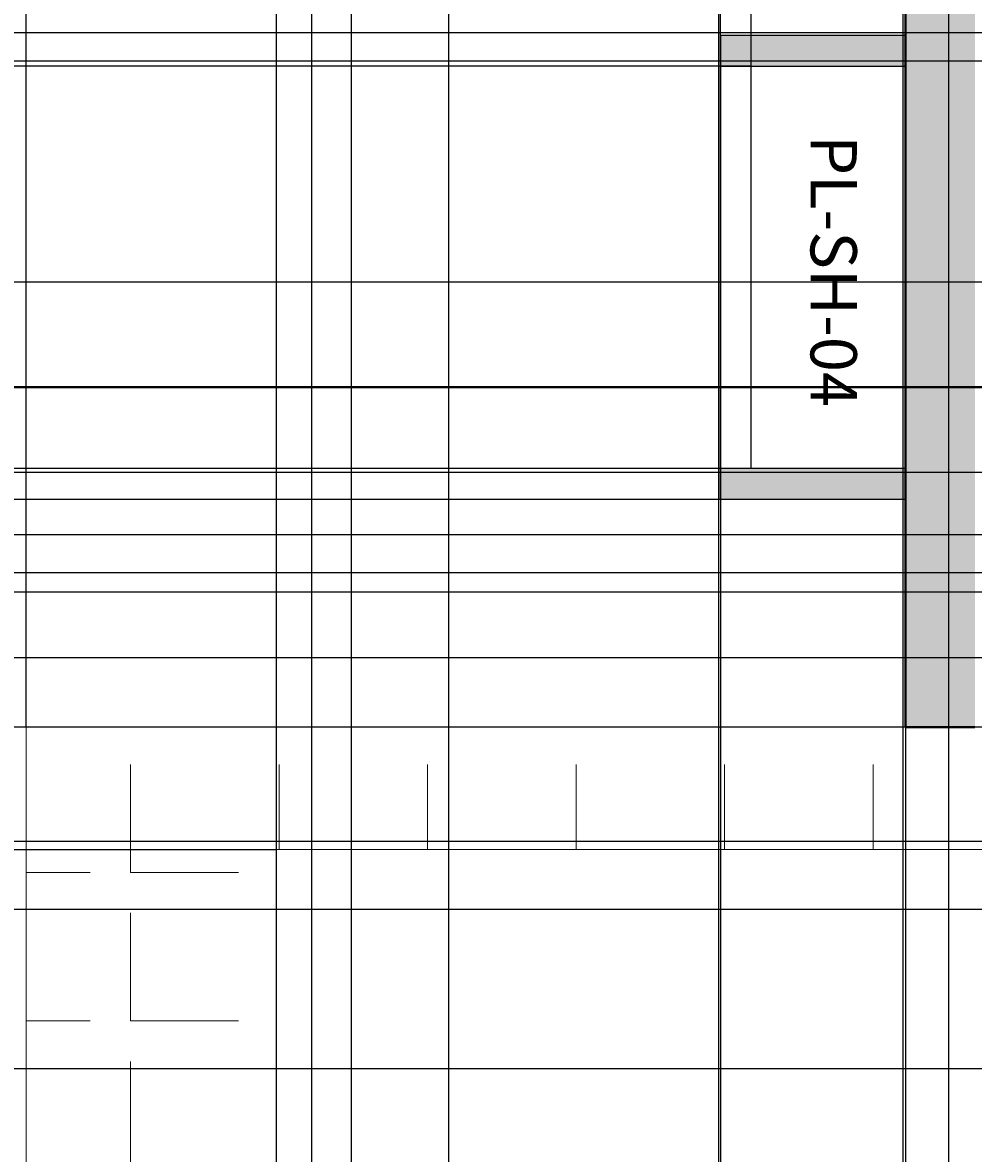
# Model space of a CAD drawing. Units: inches. Extents: x 818 to 1898, y 976 to 2364.
# Tile 7 of 96: x 1083 to 1207, y 1446 to 1592. Entities that reach past the tile are written whole.
import ezdxf

# ---------------------------------------------------------------- set-up
doc = ezdxf.new("R2010")
doc.units = ezdxf.units.IN
doc.header["$LTSCALE"] = 5
doc.header["$MEASUREMENT"] = 0
for name, color, linetype, lineweight in [('A-ANNO-DIMS', 2, 'Continuous', 18), ('A-ANNO-TEXT', 7, 'Continuous', 18), ('A-FLOR-SHFT', 7, 'Continuous', 25), ('A-WALL', 7, 'Continuous', 40), ('C-PKNG', 8, 'Continuous', 18), ('C-PKNG-PATT', 9, 'Continuous', 9), ('L-PLNT-BEDS', 94, 'Continuous', 18)]:
    doc.layers.add(name, color=color, linetype=linetype, lineweight=lineweight)
doc.layers.add('A-WALL-PATT', color=251, linetype='Continuous', lineweight=13, true_color=0x636466)
doc.styles.get("Standard").update_dxf_attribs({"font": 'arial.ttf'})
doc.dimstyles.get("Standard").update_dxf_attribs({"dimtxt": 0.18, "dimasz": 0.18, "dimexe": 0.18, "dimexo": 0.0625, "dimgap": 0.09, "dimtad": 0, "dimtih": 1, "dimtoh": 1, "dimdec": 4, "dimzin": 0, "dimdsep": 46, "dimtxsty": 'Standard', "dimcen": 0.09, "dimadec": 0, "dimazin": 0, "dimtfac": 1, "dimtdec": 4, "dimtofl": 0, "dimtmove": 0, "dimatfit": 3, "dimfxl": 1, "dimtolj": 1, "dimtzin": 0, "dimarcsym": 0})
pattern_1 = [(0, (0, 0), (0, 19.25), [14, -5.25]), (90, (0, 0), (-19.25, 1e-15), [14, -5.25])]

# ---------------------------------------------------------------- blocks, each defined once
blk = doc.blocks.new('*D59')
at = {"layer": 'A-ANNO-DIMS', "color": 0, "lineweight": -2, "ltscale": 5, "transparency": 16777216}
for p, q in [((1251.64, 2300.39), (818.03, 2300.39)), ((818.21, 2300.21), (818.21, 1669.95)), ((818.21, 1039.32), (818.21, 1669.59)), ((896.05, 1039.14), (818.03, 1039.14))]:
    blk.add_line(p, q, dxfattribs=at)
at = {"layer": 'A-ANNO-DIMS', "color": 0, "ltscale": 5, "transparency": 16777216}
for points in [[(818.18, 2300.21), (818.24, 2300.21), (818.21, 2300.39)], [(818.18, 1039.32), (818.24, 1039.32), (818.21, 1039.14)]]:
    blk.add_solid(points, dxfattribs=at)
at = {"layer": 'Defpoints', "color": 0, "ltscale": 5, "transparency": 16777216}
for p in [(818.21, 2300.39), (1251.71, 2300.39), (896.11, 1039.14)]:
    blk.add_point(p, dxfattribs=at)
at = {"layer": 'A-ANNO-DIMS', "color": 0, "ltscale": 5, "transparency": 16777216, "insert": (818.21, 1669.77), "char_height": 0.18, "attachment_point": 5}
blk.add_mtext('\\A1;1261.2', dxfattribs=at)
blk = doc.blocks.new('*D61')
at = {"layer": 'A-ANNO-DIMS', "color": 0, "lineweight": -2, "ltscale": 5, "transparency": 16777216}
for p, q in [((1071.73, 1203.03), (1071.73, 2363.87)), ((1071.91, 2363.69), (1250.94, 2363.69)), ((1430.55, 2363.69), (1251.51, 2363.69)), ((1430.73, 1203.03), (1430.73, 2363.87))]:
    blk.add_line(p, q, dxfattribs=at)
at = {"layer": 'A-ANNO-DIMS', "color": 0, "ltscale": 5, "transparency": 16777216}
for points in [[(1071.91, 2363.72), (1071.91, 2363.66), (1071.73, 2363.69)], [(1430.55, 2363.72), (1430.55, 2363.66), (1430.73, 2363.69)]]:
    blk.add_solid(points, dxfattribs=at)
at = {"layer": 'Defpoints', "color": 0, "ltscale": 5, "transparency": 16777216}
for p in [(1430.73, 2363.69), (1071.73, 1202.96), (1430.73, 1202.96)]:
    blk.add_point(p, dxfattribs=at)
at = {"layer": 'A-ANNO-DIMS', "color": 0, "ltscale": 5, "transparency": 16777216, "insert": (1251.23, 2363.69), "char_height": 0.18, "attachment_point": 5}
blk.add_mtext('\\A1;359', dxfattribs=at)
blk = doc.blocks.new('*D63')
at = {"layer": 'A-ANNO-DIMS', "color": 0, "lineweight": -2, "ltscale": 5, "transparency": 16777216}
for p, q in [((1116.13, 1485.2), (818.03, 1485.2)), ((818.21, 1485.02), (818.21, 1360.77)), ((818.21, 1236.14), (818.21, 1360.4)), ((1116.13, 1235.96), (818.03, 1235.96))]:
    blk.add_line(p, q, dxfattribs=at)
at = {"layer": 'A-ANNO-DIMS', "color": 0, "ltscale": 5, "transparency": 16777216}
for points in [[(818.18, 1485.02), (818.24, 1485.02), (818.21, 1485.2)], [(818.18, 1236.14), (818.24, 1236.14), (818.21, 1235.96)]]:
    blk.add_solid(points, dxfattribs=at)
at = {"layer": 'Defpoints', "color": 0, "ltscale": 5, "transparency": 16777216}
for p in [(818.21, 1485.2), (1116.19, 1485.2), (1116.19, 1235.96)]:
    blk.add_point(p, dxfattribs=at)
at = {"layer": 'A-ANNO-DIMS', "color": 0, "ltscale": 5, "transparency": 16777216, "insert": (818.21, 1360.58), "char_height": 0.18, "attachment_point": 5}
blk.add_mtext('\\A1;249.24', dxfattribs=at)
blk = doc.blocks.new('*D64')
at = {"layer": 'A-ANNO-DIMS', "color": 0, "lineweight": -2, "ltscale": 5, "transparency": 16777216}
for p, q in [((1197.73, 1501.14), (1197.73, 2363.87)), ((1197.91, 2363.69), (1313.93, 2363.69)), ((1430.55, 2363.69), (1314.52, 2363.69)), ((1430.73, 1501.14), (1430.73, 2363.87))]:
    blk.add_line(p, q, dxfattribs=at)
at = {"layer": 'A-ANNO-DIMS', "color": 0, "ltscale": 5, "transparency": 16777216}
for points in [[(1197.91, 2363.72), (1197.91, 2363.66), (1197.73, 2363.69)], [(1430.55, 2363.72), (1430.55, 2363.66), (1430.73, 2363.69)]]:
    blk.add_solid(points, dxfattribs=at)
at = {"layer": 'Defpoints', "color": 0, "ltscale": 5, "transparency": 16777216}
for p in [(1430.73, 2363.69), (1197.73, 1501.08), (1430.73, 1501.08)]:
    blk.add_point(p, dxfattribs=at)
at = {"layer": 'A-ANNO-DIMS', "color": 0, "ltscale": 5, "transparency": 16777216, "insert": (1314.23, 2363.69), "char_height": 0.18, "attachment_point": 5}
blk.add_mtext('\\A1;233', dxfattribs=at)
blk = doc.blocks.new('*D82')
at = {"layer": 'A-ANNO-DIMS', "color": 0, "lineweight": -2, "ltscale": 5, "transparency": 16777216}
for p, q in [((1083.73, 1501.14), (1083.73, 2363.87)), ((1083.91, 2363.69), (1140.45, 2363.69)), ((1197.55, 2363.69), (1141.01, 2363.69)), ((1197.73, 1501.14), (1197.73, 2363.87))]:
    blk.add_line(p, q, dxfattribs=at)
at = {"layer": 'A-ANNO-DIMS', "color": 0, "ltscale": 5, "transparency": 16777216}
for points in [[(1083.91, 2363.72), (1083.91, 2363.66), (1083.73, 2363.69)], [(1197.55, 2363.72), (1197.55, 2363.66), (1197.73, 2363.69)]]:
    blk.add_solid(points, dxfattribs=at)
at = {"layer": 'Defpoints', "color": 0, "ltscale": 5, "transparency": 16777216}
for p in [(1197.73, 2363.69), (1083.73, 1501.08), (1197.73, 1501.08)]:
    blk.add_point(p, dxfattribs=at)
at = {"layer": 'A-ANNO-DIMS', "color": 0, "ltscale": 5, "transparency": 16777216, "insert": (1140.73, 2363.69), "char_height": 0.18, "attachment_point": 5}
blk.add_mtext('\\A1;114', dxfattribs=at)
blk = doc.blocks.new('*D84')
at = {"layer": 'A-ANNO-DIMS', "color": 0, "lineweight": -2, "ltscale": 5, "transparency": 16777216}
for p, q in [((1197.66, 1700.08), (818.03, 1700.08)), ((818.21, 1699.9), (818.21, 1600.76)), ((818.21, 1501.26), (818.21, 1600.4)), ((1197.66, 1501.08), (818.03, 1501.08))]:
    blk.add_line(p, q, dxfattribs=at)
at = {"layer": 'A-ANNO-DIMS', "color": 0, "ltscale": 5, "transparency": 16777216}
for points in [[(818.18, 1699.9), (818.24, 1699.9), (818.21, 1700.08)], [(818.18, 1501.26), (818.24, 1501.26), (818.21, 1501.08)]]:
    blk.add_solid(points, dxfattribs=at)
at = {"layer": 'Defpoints', "color": 0, "ltscale": 5, "transparency": 16777216}
for p in [(818.21, 1700.08), (1197.73, 1700.08), (1197.73, 1501.08)]:
    blk.add_point(p, dxfattribs=at)
at = {"layer": 'A-ANNO-DIMS', "color": 0, "ltscale": 5, "transparency": 16777216, "insert": (818.21, 1600.58), "char_height": 0.18, "attachment_point": 5}
blk.add_mtext('\\A1;199', dxfattribs=at)
blk = doc.blocks.new('*D93')
at = {"layer": 'A-ANNO-DIMS', "color": 0, "lineweight": -2, "ltscale": 5, "transparency": 16777216}
for p, q in [((1068.34, 1071.12), (1068.34, 2363.87)), ((1068.52, 2363.69), (1094.16, 2363.69)), ((1120.58, 2363.69), (1094.94, 2363.69)), ((1120.76, 1071.12), (1120.76, 2363.87))]:
    blk.add_line(p, q, dxfattribs=at)
at = {"layer": 'A-ANNO-DIMS', "color": 0, "ltscale": 5, "transparency": 16777216}
for points in [[(1068.52, 2363.72), (1068.52, 2363.66), (1068.34, 2363.69)], [(1120.58, 2363.72), (1120.58, 2363.66), (1120.76, 2363.69)]]:
    blk.add_solid(points, dxfattribs=at)
at = {"layer": 'Defpoints', "color": 0, "ltscale": 5, "transparency": 16777216}
for p in [(1120.76, 2363.69), (1068.34, 1071.06), (1120.76, 1071.06)]:
    blk.add_point(p, dxfattribs=at)
at = {"layer": 'A-ANNO-DIMS', "color": 0, "ltscale": 5, "transparency": 16777216, "insert": (1094.55, 2363.69), "char_height": 0.18, "attachment_point": 5}
blk.add_mtext('\\A1;52.42', dxfattribs=at)
blk = doc.blocks.new('*D94')
at = {"layer": 'A-ANNO-DIMS', "color": 0, "lineweight": -2, "ltscale": 5, "transparency": 16777216}
for p, q in [((1120.76, 1071.12), (1120.76, 2363.87)), ((1120.94, 2363.69), (1146.76, 2363.69)), ((1173.36, 2363.69), (1147.55, 2363.69)), ((1173.54, 1071.12), (1173.54, 2363.87))]:
    blk.add_line(p, q, dxfattribs=at)
at = {"layer": 'A-ANNO-DIMS', "color": 0, "ltscale": 5, "transparency": 16777216}
for points in [[(1120.94, 2363.72), (1120.94, 2363.66), (1120.76, 2363.69)], [(1173.36, 2363.72), (1173.36, 2363.66), (1173.54, 2363.69)]]:
    blk.add_solid(points, dxfattribs=at)
at = {"layer": 'Defpoints', "color": 0, "ltscale": 5, "transparency": 16777216}
for p in [(1173.54, 2363.69), (1120.76, 1071.06), (1173.54, 1071.06)]:
    blk.add_point(p, dxfattribs=at)
at = {"layer": 'A-ANNO-DIMS', "color": 0, "ltscale": 5, "transparency": 16777216, "insert": (1147.15, 2363.69), "char_height": 0.18, "attachment_point": 5}
blk.add_mtext('\\A1;52.78', dxfattribs=at)
blk = doc.blocks.new('*D95')
at = {"layer": 'A-ANNO-DIMS', "color": 0, "lineweight": -2, "ltscale": 5, "transparency": 16777216}
for p, q in [((1173.54, 1071.12), (1173.54, 2363.87)), ((1173.72, 2363.69), (1201.29, 2363.69)), ((1229.47, 2363.69), (1201.9, 2363.69)), ((1229.65, 1071.12), (1229.65, 2363.87))]:
    blk.add_line(p, q, dxfattribs=at)
at = {"layer": 'A-ANNO-DIMS', "color": 0, "ltscale": 5, "transparency": 16777216}
for points in [[(1173.72, 2363.72), (1173.72, 2363.66), (1173.54, 2363.69)], [(1229.47, 2363.72), (1229.47, 2363.66), (1229.65, 2363.69)]]:
    blk.add_solid(points, dxfattribs=at)
at = {"layer": 'Defpoints', "color": 0, "ltscale": 5, "transparency": 16777216}
for p in [(1229.65, 2363.69), (1173.54, 1071.06), (1229.65, 1071.06)]:
    blk.add_point(p, dxfattribs=at)
at = {"layer": 'A-ANNO-DIMS', "color": 0, "ltscale": 5, "transparency": 16777216, "insert": (1201.59, 2363.69), "char_height": 0.18, "attachment_point": 5}
blk.add_mtext('\\A1;56.1', dxfattribs=at)
blk = doc.blocks.new('*D109')
at = {"layer": 'A-ANNO-DIMS', "color": 0, "lineweight": -2, "ltscale": 5, "transparency": 16777216}
for p, q in [((1125.92, 1410.12), (1125.92, 2363.87)), ((1126.1, 2363.69), (1164.25, 2363.69)), ((1203.15, 2363.69), (1165, 2363.69)), ((1203.33, 1409.91), (1203.33, 2363.87))]:
    blk.add_line(p, q, dxfattribs=at)
at = {"layer": 'A-ANNO-DIMS', "color": 0, "ltscale": 5, "transparency": 16777216}
for points in [[(1126.1, 2363.72), (1126.1, 2363.66), (1125.92, 2363.69)], [(1203.15, 2363.72), (1203.15, 2363.66), (1203.33, 2363.69)]]:
    blk.add_solid(points, dxfattribs=at)
at = {"layer": 'Defpoints', "color": 0, "ltscale": 5, "transparency": 16777216}
for p in [(1203.33, 2363.69), (1125.92, 1410.05), (1203.33, 1409.85)]:
    blk.add_point(p, dxfattribs=at)
at = {"layer": 'A-ANNO-DIMS', "color": 0, "ltscale": 5, "transparency": 16777216, "insert": (1164.62, 2363.69), "char_height": 0.18, "attachment_point": 5}
blk.add_mtext('\\A1;77.41', dxfattribs=at)
blk = doc.blocks.new('*D116')
at = {"layer": 'A-ANNO-DIMS', "color": 0, "lineweight": -2, "ltscale": 5, "transparency": 16777216}
for p, q in [((1766.29, 1456.81), (818.03, 1456.81)), ((818.21, 1456.63), (818.21, 1417.41)), ((818.21, 1377.84), (818.21, 1417.05)), ((1766.29, 1377.66), (818.03, 1377.66))]:
    blk.add_line(p, q, dxfattribs=at)
at = {"layer": 'A-ANNO-DIMS', "color": 0, "ltscale": 5, "transparency": 16777216}
for points in [[(818.18, 1456.63), (818.24, 1456.63), (818.21, 1456.81)], [(818.18, 1377.84), (818.24, 1377.84), (818.21, 1377.66)]]:
    blk.add_solid(points, dxfattribs=at)
at = {"layer": 'Defpoints', "color": 0, "ltscale": 5, "transparency": 16777216}
for p in [(818.21, 1456.81), (1766.35, 1456.81), (1766.35, 1377.66)]:
    blk.add_point(p, dxfattribs=at)
at = {"layer": 'A-ANNO-DIMS', "color": 0, "ltscale": 5, "transparency": 16777216, "insert": (818.21, 1417.23), "char_height": 0.18, "attachment_point": 5}
blk.add_mtext('\\A1;79.15', dxfattribs=at)
blk = doc.blocks.new('*D117')
at = {"layer": 'A-ANNO-DIMS', "color": 0, "lineweight": -2, "ltscale": 5, "transparency": 16777216}
for p, q in [((1766.29, 1545.18), (818.03, 1545.18)), ((818.21, 1545), (818.21, 1501.18)), ((818.21, 1456.99), (818.21, 1500.81)), ((1766.29, 1456.81), (818.03, 1456.81))]:
    blk.add_line(p, q, dxfattribs=at)
at = {"layer": 'A-ANNO-DIMS', "color": 0, "ltscale": 5, "transparency": 16777216}
for points in [[(818.18, 1545), (818.24, 1545), (818.21, 1545.18)], [(818.18, 1456.99), (818.24, 1456.99), (818.21, 1456.81)]]:
    blk.add_solid(points, dxfattribs=at)
at = {"layer": 'Defpoints', "color": 0, "ltscale": 5, "transparency": 16777216}
for p in [(818.21, 1545.18), (1766.35, 1545.18), (1766.35, 1456.81)]:
    blk.add_point(p, dxfattribs=at)
at = {"layer": 'A-ANNO-DIMS', "color": 0, "ltscale": 5, "transparency": 16777216, "insert": (818.21, 1501), "char_height": 0.18, "attachment_point": 5}
blk.add_mtext('\\A1;88.37', dxfattribs=at)
blk = doc.blocks.new('*D118')
at = {"layer": 'A-ANNO-DIMS', "color": 0, "lineweight": -2, "ltscale": 5, "transparency": 16777216}
for p, q in [((1766.29, 1627.51), (818.03, 1627.51)), ((818.21, 1627.33), (818.21, 1586.53)), ((818.21, 1545.36), (818.21, 1586.16)), ((1766.29, 1545.18), (818.03, 1545.18))]:
    blk.add_line(p, q, dxfattribs=at)
at = {"layer": 'A-ANNO-DIMS', "color": 0, "ltscale": 5, "transparency": 16777216}
for points in [[(818.18, 1627.33), (818.24, 1627.33), (818.21, 1627.51)], [(818.18, 1545.36), (818.24, 1545.36), (818.21, 1545.18)]]:
    blk.add_solid(points, dxfattribs=at)
at = {"layer": 'Defpoints', "color": 0, "ltscale": 5, "transparency": 16777216}
for p in [(818.21, 1627.51), (1766.35, 1627.51), (1766.35, 1545.18)]:
    blk.add_point(p, dxfattribs=at)
at = {"layer": 'A-ANNO-DIMS', "color": 0, "ltscale": 5, "transparency": 16777216, "insert": (818.21, 1586.34), "char_height": 0.18, "attachment_point": 5}
blk.add_mtext('\\A1;82.32', dxfattribs=at)
blk = doc.blocks.new('*D122')
at = {"layer": 'A-ANNO-DIMS', "color": 0, "lineweight": -2, "ltscale": 5, "transparency": 16777216}
for p, q in [((1138.5, 1794.37), (1138.5, 975.66)), ((1071.73, 1688.02), (1071.73, 975.66)), ((1071.91, 975.84), (1104.72, 975.84)), ((1138.32, 975.84), (1105.51, 975.84))]:
    blk.add_line(p, q, dxfattribs=at)
at = {"layer": 'A-ANNO-DIMS', "color": 0, "ltscale": 5, "transparency": 16777216}
for points in [[(1071.91, 975.87), (1071.91, 975.81), (1071.73, 975.84)], [(1138.32, 975.87), (1138.32, 975.81), (1138.5, 975.84)]]:
    blk.add_solid(points, dxfattribs=at)
at = {"layer": 'Defpoints', "color": 0, "ltscale": 5, "transparency": 16777216}
for p in [(1138.5, 1794.43), (1071.73, 1688.08), (1138.5, 975.84)]:
    blk.add_point(p, dxfattribs=at)
at = {"layer": 'A-ANNO-DIMS', "color": 0, "ltscale": 5, "transparency": 16777216, "insert": (1105.11, 975.84), "char_height": 0.18, "attachment_point": 5}
blk.add_mtext('\\A1;66.78', dxfattribs=at)
blk = doc.blocks.new('*D126')
at = {"layer": 'A-ANNO-DIMS', "color": 0, "lineweight": -2, "ltscale": 5, "transparency": 16777216}
for p, q in [((1035.38, 1252.09), (1035.38, 2363.87)), ((1035.56, 2363.69), (1075.41, 2363.69)), ((1116.01, 2363.69), (1076.16, 2363.69)), ((1116.19, 1236.03), (1116.19, 2363.87))]:
    blk.add_line(p, q, dxfattribs=at)
at = {"layer": 'A-ANNO-DIMS', "color": 0, "ltscale": 5, "transparency": 16777216}
for points in [[(1035.56, 2363.72), (1035.56, 2363.66), (1035.38, 2363.69)], [(1116.01, 2363.72), (1116.01, 2363.66), (1116.19, 2363.69)]]:
    blk.add_solid(points, dxfattribs=at)
at = {"layer": 'Defpoints', "color": 0, "ltscale": 5, "transparency": 16777216}
for p in [(1035.38, 2363.69), (1035.38, 1252.02), (1116.19, 1235.96)]:
    blk.add_point(p, dxfattribs=at)
at = {"layer": 'A-ANNO-DIMS', "color": 0, "ltscale": 5, "transparency": 16777216, "insert": (1075.78, 2363.69), "char_height": 0.18, "attachment_point": 5}
blk.add_mtext('\\A1;80.81', dxfattribs=at)
blk = doc.blocks.new('*D145')
at = {"layer": 'A-ANNO-DIMS', "color": 0, "lineweight": -2, "ltscale": 5, "transparency": 16777216}
for p, q in [((1197.39, 2122.31), (1197.39, 975.66)), ((1232.61, 2122.31), (1232.61, 975.66)), ((1197.57, 975.84), (1214.61, 975.84)), ((1232.43, 975.84), (1215.39, 975.84))]:
    blk.add_line(p, q, dxfattribs=at)
at = {"layer": 'A-ANNO-DIMS', "color": 0, "ltscale": 5, "transparency": 16777216}
for points in [[(1197.57, 975.87), (1197.57, 975.81), (1197.39, 975.84)], [(1232.43, 975.87), (1232.43, 975.81), (1232.61, 975.84)]]:
    blk.add_solid(points, dxfattribs=at)
at = {"layer": 'Defpoints', "color": 0, "ltscale": 5, "transparency": 16777216}
for p in [(1197.39, 2122.38), (1232.61, 2122.38), (1232.61, 975.84)]:
    blk.add_point(p, dxfattribs=at)
at = {"layer": 'A-ANNO-DIMS', "color": 0, "ltscale": 5, "transparency": 16777216, "insert": (1215, 975.84), "char_height": 0.18, "attachment_point": 5}
blk.add_mtext('\\A1;35.22', dxfattribs=at)
blk = doc.blocks.new('*D155')
at = {"layer": 'A-ANNO-DIMS', "color": 0, "lineweight": -2, "ltscale": 5, "transparency": 16777216}
for p, q in [((1173.73, 1590.7), (1173.73, 975.66)), ((1197.73, 1530.54), (1197.73, 975.66)), ((1173.91, 975.84), (1185.51, 975.84)), ((1197.55, 975.84), (1185.95, 975.84))]:
    blk.add_line(p, q, dxfattribs=at)
at = {"layer": 'A-ANNO-DIMS', "color": 0, "ltscale": 5, "transparency": 16777216}
for points in [[(1173.91, 975.87), (1173.91, 975.81), (1173.73, 975.84)], [(1197.55, 975.87), (1197.55, 975.81), (1197.73, 975.84)]]:
    blk.add_solid(points, dxfattribs=at)
at = {"layer": 'Defpoints', "color": 0, "ltscale": 5, "transparency": 16777216}
for p in [(1173.73, 1590.76), (1197.73, 1530.6), (1173.73, 975.84)]:
    blk.add_point(p, dxfattribs=at)
at = {"layer": 'A-ANNO-DIMS', "color": 0, "ltscale": 5, "transparency": 16777216, "insert": (1185.73, 975.84), "char_height": 0.18, "attachment_point": 5}
blk.add_mtext('\\A1;24', dxfattribs=at)
blk = doc.blocks.new('*D156')
at = {"layer": 'A-ANNO-DIMS', "color": 0, "lineweight": -2, "ltscale": 5, "transparency": 16777216}
for p, q in [((1177.66, 1586.76), (818.03, 1586.76)), ((818.21, 1586.58), (818.21, 1560.86)), ((818.21, 1534.78), (818.21, 1560.5)), ((1177.66, 1534.6), (818.03, 1534.6))]:
    blk.add_line(p, q, dxfattribs=at)
at = {"layer": 'A-ANNO-DIMS', "color": 0, "ltscale": 5, "transparency": 16777216}
for points in [[(818.18, 1586.58), (818.24, 1586.58), (818.21, 1586.76)], [(818.18, 1534.78), (818.24, 1534.78), (818.21, 1534.6)]]:
    blk.add_solid(points, dxfattribs=at)
at = {"layer": 'Defpoints', "color": 0, "ltscale": 5, "transparency": 16777216}
for p in [(818.21, 1586.76), (1177.73, 1586.76), (1177.73, 1534.6)]:
    blk.add_point(p, dxfattribs=at)
at = {"layer": 'A-ANNO-DIMS', "color": 0, "ltscale": 5, "transparency": 16777216, "insert": (818.21, 1560.68), "char_height": 0.18, "attachment_point": 5}
blk.add_mtext('\\A1;52.16', dxfattribs=at)
blk = doc.blocks.new('*D157')
at = {"layer": 'A-ANNO-DIMS', "color": 0, "lineweight": -2, "ltscale": 5, "transparency": 16777216}
for p, q in [((1197.66, 1530.6), (818.03, 1530.6)), ((818.21, 1530.42), (818.21, 1516.02)), ((818.21, 1501.26), (818.21, 1515.66)), ((1197.66, 1501.08), (818.03, 1501.08))]:
    blk.add_line(p, q, dxfattribs=at)
at = {"layer": 'A-ANNO-DIMS', "color": 0, "ltscale": 5, "transparency": 16777216}
for points in [[(818.18, 1530.42), (818.24, 1530.42), (818.21, 1530.6)], [(818.18, 1501.26), (818.24, 1501.26), (818.21, 1501.08)]]:
    blk.add_solid(points, dxfattribs=at)
at = {"layer": 'Defpoints', "color": 0, "ltscale": 5, "transparency": 16777216}
for p in [(818.21, 1530.6), (1197.73, 1530.6), (1197.73, 1501.08)]:
    blk.add_point(p, dxfattribs=at)
at = {"layer": 'A-ANNO-DIMS', "color": 0, "ltscale": 5, "transparency": 16777216, "insert": (818.21, 1515.84), "char_height": 0.18, "attachment_point": 5}
blk.add_mtext('\\A1;29.524', dxfattribs=at)
blk = doc.blocks.new('*D158')
at = {"layer": 'A-ANNO-DIMS', "color": 0, "lineweight": -2, "ltscale": 5, "transparency": 16777216}
for p, q in [((1173.73, 1590.82), (1173.73, 2363.87)), ((1173.91, 2363.69), (1175.57, 2363.69)), ((1177.55, 2363.69), (1175.88, 2363.69)), ((1177.73, 1586.82), (1177.73, 2363.87))]:
    blk.add_line(p, q, dxfattribs=at)
at = {"layer": 'A-ANNO-DIMS', "color": 0, "ltscale": 5, "transparency": 16777216}
for points in [[(1173.91, 2363.72), (1173.91, 2363.66), (1173.73, 2363.69)], [(1177.55, 2363.72), (1177.55, 2363.66), (1177.73, 2363.69)]]:
    blk.add_solid(points, dxfattribs=at)
at = {"layer": 'Defpoints', "color": 0, "ltscale": 5, "transparency": 16777216}
for p in [(1177.73, 2363.69), (1173.73, 1590.76), (1177.73, 1586.76)]:
    blk.add_point(p, dxfattribs=at)
at = {"layer": 'A-ANNO-DIMS', "color": 0, "ltscale": 5, "transparency": 16777216, "insert": (1175.73, 2363.69), "char_height": 0.18, "attachment_point": 5}
blk.add_mtext('\\A1;4', dxfattribs=at)
blk = doc.blocks.new('*D168')
at = {"layer": 'A-ANNO-DIMS', "color": 0, "lineweight": -2, "ltscale": 5, "transparency": 16777216}
for p, q in [((1430.66, 1501.08), (818.03, 1501.08)), ((818.21, 1500.9), (818.21, 1493.84)), ((818.21, 1486.42), (818.21, 1493.48)), ((1430.66, 1486.24), (818.03, 1486.24))]:
    blk.add_line(p, q, dxfattribs=at)
at = {"layer": 'A-ANNO-DIMS', "color": 0, "ltscale": 5, "transparency": 16777216}
for points in [[(818.18, 1500.9), (818.24, 1500.9), (818.21, 1501.08)], [(818.18, 1486.42), (818.24, 1486.42), (818.21, 1486.24)]]:
    blk.add_solid(points, dxfattribs=at)
at = {"layer": 'Defpoints', "color": 0, "ltscale": 5, "transparency": 16777216}
for p in [(818.21, 1501.08), (1430.73, 1501.08), (1430.73, 1486.24)]:
    blk.add_point(p, dxfattribs=at)
at = {"layer": 'A-ANNO-DIMS', "color": 0, "ltscale": 5, "transparency": 16777216, "insert": (818.21, 1493.66), "char_height": 0.18, "attachment_point": 5}
blk.add_mtext('\\A1;14.84', dxfattribs=at)
blk = doc.blocks.new('*D187')
at = {"layer": 'A-ANNO-DIMS', "color": 0, "lineweight": -2, "ltscale": 5, "transparency": 16777216}
for p, q in [((1705.66, 1545.08), (818.03, 1545.08)), ((818.21, 1544.9), (818.21, 1533.26)), ((818.21, 1521.26), (818.21, 1532.9)), ((1705.66, 1521.08), (818.03, 1521.08))]:
    blk.add_line(p, q, dxfattribs=at)
at = {"layer": 'A-ANNO-DIMS', "color": 0, "ltscale": 5, "transparency": 16777216}
for points in [[(818.18, 1544.9), (818.24, 1544.9), (818.21, 1545.08)], [(818.18, 1521.26), (818.24, 1521.26), (818.21, 1521.08)]]:
    blk.add_solid(points, dxfattribs=at)
at = {"layer": 'Defpoints', "color": 0, "ltscale": 5, "transparency": 16777216}
for p in [(818.21, 1545.08), (1705.73, 1545.08), (1705.73, 1521.08)]:
    blk.add_point(p, dxfattribs=at)
at = {"layer": 'A-ANNO-DIMS', "color": 0, "ltscale": 5, "transparency": 16777216, "insert": (818.21, 1533.08), "char_height": 0.18, "attachment_point": 5}
blk.add_mtext('\\A1;24', dxfattribs=at)
blk = doc.blocks.new('*D194')
at = {"layer": 'A-ANNO-DIMS', "color": 0, "lineweight": -2, "ltscale": 5, "transparency": 16777216}
for p, q in [((1616.66, 1591.08), (818.03, 1591.08)), ((818.21, 1590.9), (818.21, 1575.1)), ((818.21, 1558.93), (818.21, 1574.73)), ((1616.66, 1558.75), (818.03, 1558.75))]:
    blk.add_line(p, q, dxfattribs=at)
at = {"layer": 'A-ANNO-DIMS', "color": 0, "ltscale": 5, "transparency": 16777216}
for points in [[(818.18, 1590.9), (818.24, 1590.9), (818.21, 1591.08)], [(818.18, 1558.93), (818.24, 1558.93), (818.21, 1558.75)]]:
    blk.add_solid(points, dxfattribs=at)
at = {"layer": 'Defpoints', "color": 0, "ltscale": 5, "transparency": 16777216}
for p in [(818.21, 1591.08), (1616.73, 1591.08), (1616.73, 1558.75)]:
    blk.add_point(p, dxfattribs=at)
at = {"layer": 'A-ANNO-DIMS', "color": 0, "ltscale": 5, "transparency": 16777216, "insert": (818.21, 1574.92), "char_height": 0.18, "attachment_point": 5}
blk.add_mtext('\\A1;32.326', dxfattribs=at)
blk = doc.blocks.new('*D201')
at = {"layer": 'A-ANNO-DIMS', "color": 0, "lineweight": -2, "ltscale": 5, "transparency": 16777216}
for p, q in [((1678.27, 1518.56), (818.03, 1518.56)), ((818.21, 1518.38), (818.21, 1498.18)), ((818.21, 1477.61), (818.21, 1497.81)), ((1678.27, 1477.43), (818.03, 1477.43))]:
    blk.add_line(p, q, dxfattribs=at)
at = {"layer": 'A-ANNO-DIMS', "color": 0, "ltscale": 5, "transparency": 16777216}
for points in [[(818.18, 1518.38), (818.24, 1518.38), (818.21, 1518.56)], [(818.18, 1477.61), (818.24, 1477.61), (818.21, 1477.43)]]:
    blk.add_solid(points, dxfattribs=at)
at = {"layer": 'Defpoints', "color": 0, "ltscale": 5, "transparency": 16777216}
for p in [(818.21, 1518.56), (1678.33, 1518.56), (1678.33, 1477.43)]:
    blk.add_point(p, dxfattribs=at)
at = {"layer": 'A-ANNO-DIMS', "color": 0, "ltscale": 5, "transparency": 16777216, "insert": (818.21, 1497.99), "char_height": 0.18, "attachment_point": 5}
blk.add_mtext('\\A1;41.135', dxfattribs=at)
blk = doc.blocks.new('*D270')
at = {"layer": 'A-ANNO-DIMS', "color": 0, "lineweight": -2, "ltscale": 5, "transparency": 16777216}
for p, q in [((1246.88, 1534.08), (818.03, 1534.08)), ((818.21, 1533.9), (818.21, 1522.26)), ((818.21, 1510.26), (818.21, 1521.9)), ((1246.88, 1510.08), (818.03, 1510.08))]:
    blk.add_line(p, q, dxfattribs=at)
at = {"layer": 'A-ANNO-DIMS', "color": 0, "ltscale": 5, "transparency": 16777216}
for points in [[(818.18, 1533.9), (818.24, 1533.9), (818.21, 1534.08)], [(818.18, 1510.26), (818.24, 1510.26), (818.21, 1510.08)]]:
    blk.add_solid(points, dxfattribs=at)
at = {"layer": 'Defpoints', "color": 0, "ltscale": 5, "transparency": 16777216}
for p in [(818.21, 1534.08), (1246.94, 1534.08), (1246.94, 1510.08)]:
    blk.add_point(p, dxfattribs=at)
at = {"layer": 'A-ANNO-DIMS', "color": 0, "ltscale": 5, "transparency": 16777216, "insert": (818.21, 1522.08), "char_height": 0.18, "attachment_point": 5}
blk.add_mtext('\\A1;24', dxfattribs=at)
blk = doc.blocks.new('*D272')
at = {"layer": 'A-ANNO-DIMS', "color": 0, "lineweight": -2, "ltscale": 5, "transparency": 16777216}
for p, q in [((1406.66, 1587.42), (818.03, 1587.42)), ((818.21, 1587.24), (818.21, 1556.89)), ((818.21, 1526.18), (818.21, 1556.52)), ((1406.66, 1526), (818.03, 1526))]:
    blk.add_line(p, q, dxfattribs=at)
at = {"layer": 'A-ANNO-DIMS', "color": 0, "ltscale": 5, "transparency": 16777216}
for points in [[(818.18, 1587.24), (818.24, 1587.24), (818.21, 1587.42)], [(818.18, 1526.18), (818.24, 1526.18), (818.21, 1526)]]:
    blk.add_solid(points, dxfattribs=at)
at = {"layer": 'Defpoints', "color": 0, "ltscale": 5, "transparency": 16777216}
for p in [(818.21, 1587.42), (1406.73, 1587.42), (1406.73, 1526)]:
    blk.add_point(p, dxfattribs=at)
at = {"layer": 'A-ANNO-DIMS', "color": 0, "ltscale": 5, "transparency": 16777216, "insert": (818.21, 1556.71), "char_height": 0.18, "attachment_point": 5}
blk.add_mtext('\\A1;61.42', dxfattribs=at)

msp = doc.modelspace()

# ---------------------------------------------------------------- hatches: boundary and pattern name
at = {"layer": 'A-WALL-PATT', "ltscale": 5}
h = msp.add_hatch(color=256, dxfattribs=at)
h.dxf.hatch_style = 1
h.paths.add_polyline_path([(1206.7252, 1687.0782), (1206.7252, 1700.0782), (1197.7251, 1700.0782), (1197.7251, 1501.0782), (1206.7252, 1501.0782), (1206.7252, 1510.0782)])
h.paths.add_polyline_path([(1197.7251, 1590.7585), (1173.7251, 1590.7585), (1173.7251, 1586.7585), (1197.7251, 1586.7585)])
h.paths.add_polyline_path([(1197.7251, 1534.6024), (1173.7251, 1534.6024), (1173.7251, 1530.6024), (1197.7251, 1530.6024)])
h.paths.add_polyline_path([(1365.1463, 1510.0782), (1283.8183, 1510.0782), (1283.8183, 1501.0782), (1365.1463, 1501.0782)])
h.paths.add_polyline_path([(1439.7252, 1591.0782), (1441.7252, 1591.0782), (1441.7252, 1600.0782), (1430.7251, 1600.0782), (1430.7251, 1510.0782), (1406.7251, 1510.0782), (1401.1463, 1510.0782), (1401.1463, 1501.0782), (1430.7251, 1501.0782), (1430.7251, 1486.2383), (1430.7251, 1409.0522), (1439.7252, 1409.0522)])
at = {"layer": 'C-PKNG-PATT', "ltscale": 5}
h = msp.add_hatch(dxfattribs=at)
h.set_pattern_fill('ANGLE', color=256, scale=70)
h.set_pattern_definition(pattern_1)
h.paths.add_polyline_path([(1430.7251, 1211.9642), (1430.7251, 1486.2383), (1406.7251, 1486.2383), (1406.7251, 1235.9642), (1116.1882, 1235.9642), (1116.1882, 1485.2035), (1345.9651, 1485.2035), (1345.9651, 1501.0782), (1206.7252, 1501.0782), (1197.7251, 1501.0782), (1083.7251, 1501.0782), (1083.7251, 1485.2035), (1083.7251, 1211.9642)])
h = msp.add_hatch(dxfattribs=at)
h.set_pattern_fill('ANGLE', color=256, scale=70)
h.set_pattern_definition(pattern_1)
h.paths.add_polyline_path([(1116.1882, 1485.2035), (1345.9651, 1485.2035), (1345.9651, 1501.0782), (1206.7252, 1501.0782), (1197.7251, 1501.0782), (1083.7251, 1501.0782), (1083.7251, 1485.2035), (1083.7251, 1211.9642), (1430.7251, 1211.9642), (1430.7251, 1271.1621), (1430.7251, 1290.0782), (1430.7251, 1346.0782), (1430.7251, 1486.2383), (1406.7251, 1486.2383), (1406.7251, 1235.9642), (1116.1882, 1235.9642)])

# ---------------------------------------------------------------- linework, layer by layer
at = {"layer": 'A-FLOR-SHFT'}
for p, q in [((1173.7251, 1530.6024), (1173.7251, 1590.7585)), ((1173.7251, 1590.7585), (1197.7251, 1590.7585)), ((1173.7251, 1586.7585), (1197.7251, 1586.7585)), ((1177.7251, 1534.6024), (1177.7251, 1586.7585)), ((1197.7251, 1534.6024), (1173.7251, 1534.6024)), ((1197.7251, 1530.6024), (1173.7251, 1530.6024))]:
    msp.add_line(p, q, dxfattribs=at)
at = {"layer": 'A-WALL'}
msp.add_line((1197.7251, 1700.0782), (1197.7251, 1501.0782), dxfattribs=at)
at = {"layer": 'A-WALL', "ltscale": 5}
msp.add_line((1206.7252, 1501.0782), (1197.7251, 1501.0782), dxfattribs=at)
at = {"layer": 'C-PKNG', "ltscale": 5}
for p, q in [((1083.7251, 1501.0782), (1083.7251, 1485.2035)), ((1197.7251, 1501.0782), (1083.7251, 1501.0782)), ((1116.1882, 1485.2035), (1116.1882, 1235.9642)), ((1116.1882, 1485.2035), (1345.9651, 1485.2035))]:
    msp.add_line(p, q, dxfattribs=at)
at = {"layer": 'L-PLNT-BEDS'}
msp.add_line((1083.7251, 2044.0782), (1083.7251, 1211.9642), dxfattribs=at)

# ---------------------------------------------------------------- texts
at = {"layer": 'A-ANNO-TEXT', "ltscale": 5, "insert": (1191.4167, 1577.8153), "char_height": 6, "attachment_point": 1, "rotation": 270}
msp.add_mtext_dynamic_manual_height_columns('PL-SH-04', width=118.992422, gutter_width=1, heights=[0], dxfattribs=at)

# ---------------------------------------------------------------- dimensions: what is measured, and where the dimension line sits
at = {"layer": 'A-ANNO-DIMS', "ltscale": 5}
for base, p1, p2, override, picture, middle in [((1035.3768, 2363.6929), (1116.1882, 1235.9642), (1035.3768, 1252.0242), {"dimdec": 2, "dimlfac": 1, "dimrnd": 0, "dimzin": 0, "dimdsep": 46, "dimlunit": 2}, '*D126', (1075.7825, 2363.6929)), ((1120.7618, 2363.6929), (1068.3377, 1071.0552), (1120.7618, 1071.0552), {"dimdec": 2, "dimlfac": 1, "dimrnd": 0, "dimzin": 0, "dimdsep": 46, "dimlunit": 2}, '*D93', (1094.5497, 2363.6929)), ((1430.7251, 2363.6929), (1071.7251, 1202.9642), (1430.7251, 1202.9642), {"dimdec": 0, "dimlfac": 1, "dimrnd": 0, "dimzin": 0, "dimdsep": 46, "dimlunit": 2}, '*D61', (1251.2251, 2363.6929)), ((1197.7251, 2363.6929), (1083.7251, 1501.0782), (1197.7251, 1501.0782), {"dimdec": 0, "dimlfac": 1, "dimrnd": 0, "dimzin": 0, "dimdsep": 46, "dimlunit": 2}, '*D82', (1140.7251, 2363.6929)), ((1173.5418, 2363.6929), (1120.7618, 1071.0552), (1173.5418, 1071.0552), {"dimdec": 2, "dimlfac": 1, "dimrnd": 0, "dimzin": 0, "dimdsep": 46, "dimlunit": 2}, '*D94', (1147.1518, 2363.6929)), ((1203.3292, 2363.6929), (1125.9172, 1410.0547), (1203.3292, 1409.8484), {"dimdec": 2, "dimlfac": 1, "dimrnd": 0, "dimzin": 0, "dimdsep": 46, "dimlunit": 2}, '*D109', (1164.6232, 2363.6929)), ((1229.6474, 2363.6929), (1173.5418, 1071.0552), (1229.6474, 1071.0552), {"dimdec": 1, "dimlfac": 1, "dimrnd": 0, "dimzin": 0, "dimdsep": 46, "dimlunit": 2}, '*D95', (1201.5946, 2363.6929)), ((1177.7251, 2363.6929), (1173.7251, 1590.7585), (1177.7251, 1586.7585), {"dimdec": 0, "dimlfac": 1, "dimrnd": 0, "dimzin": 0, "dimdsep": 46, "dimlunit": 2}, '*D158', (1175.7251, 2363.6929)), ((1430.7251, 2363.6929), (1197.7251, 1501.0782), (1430.7251, 1501.0782), {"dimdec": 0, "dimlfac": 1, "dimrnd": 0, "dimzin": 0, "dimdsep": 46, "dimlunit": 2}, '*D64', (1314.2251, 2363.6929)), ((1232.6091, 975.8433), (1197.3925, 2122.3767), (1232.6091, 2122.3767), {"dimdec": 2, "dimlfac": 1, "dimrnd": 0, "dimzin": 0, "dimdsep": 46, "dimlunit": 2}, '*D145', (1215.0008, 975.8433)), ((1138.5041, 975.8433), (1071.7251, 1688.0782), (1138.5041, 1794.4325), {"dimdec": 2, "dimlfac": 1, "dimrnd": 0, "dimzin": 0, "dimdsep": 46, "dimlunit": 2}, '*D122', (1105.1146, 975.8433)), ((1173.7251, 975.8433), (1197.7251, 1530.6024), (1173.7251, 1590.7585), {"dimdec": 0, "dimlfac": 1, "dimrnd": 0, "dimzin": 0, "dimdsep": 46, "dimlunit": 2}, '*D155', (1185.7251, 975.8433))]:
    dim = msp.add_linear_dim(base=base, p1=p1, p2=p2, dimstyle='Standard', override=override, dxfattribs=at)
    dim.commit()
    dim.dimension.update_dxf_attribs({"geometry": picture, "text_midpoint": middle})
for base, p1, p2, override, picture, middle in [((818.2059, 2300.3929), (896.1138, 1039.1433), (1251.7057, 2300.3929), {"dimdec": 1, "dimlfac": 1, "dimrnd": 0, "dimzin": 0, "dimdsep": 46, "dimlunit": 2}, '*D59', (818.2059, 1669.7681)), ((818.2059, 1700.0782), (1197.7251, 1501.0782), (1197.7251, 1700.0782), {"dimdec": 0, "dimlfac": 1, "dimrnd": 0, "dimzin": 0, "dimdsep": 46, "dimlunit": 2}, '*D84', (818.2059, 1600.5782)), ((818.2059, 1627.5052), (1766.3524, 1545.1827), (1766.3524, 1627.5052), {"dimdec": 2, "dimlfac": 1, "dimrnd": 0, "dimzin": 0, "dimdsep": 46, "dimlunit": 2}, '*D118', (818.2059, 1586.3439)), ((818.2059, 1591.0782), (1616.7251, 1558.7521), (1616.7251, 1591.0782), {"dimdec": 3, "dimlfac": 1, "dimrnd": 0, "dimzin": 0, "dimdsep": 46, "dimlunit": 2}, '*D194', (818.2059, 1574.9152)), ((818.2059, 1587.4164), (1406.7251, 1525.9965), (1406.7251, 1587.4164), {"dimdec": 2, "dimlfac": 1, "dimrnd": 0, "dimzin": 0, "dimdsep": 46, "dimlunit": 2}, '*D272', (818.2059, 1556.7064)), ((818.2059, 1586.7585), (1177.7251, 1534.6024), (1177.7251, 1586.7585), {"dimdec": 2, "dimlfac": 1, "dimrnd": 0, "dimzin": 0, "dimdsep": 46, "dimlunit": 2}, '*D156', (818.2059, 1560.6805)), ((818.2059, 1545.1827), (1766.3524, 1456.8088), (1766.3524, 1545.1827), {"dimdec": 2, "dimlfac": 1, "dimrnd": 0, "dimzin": 0, "dimdsep": 46, "dimlunit": 2}, '*D117', (818.2059, 1500.9957)), ((818.2059, 1545.0782), (1705.7251, 1521.0782), (1705.7251, 1545.0782), {"dimdec": 0, "dimlfac": 1, "dimrnd": 0, "dimzin": 0, "dimdsep": 46, "dimlunit": 2}, '*D187', (818.2059, 1533.0782)), ((818.2059, 1534.0782), (1246.9377, 1510.0782), (1246.9377, 1534.0782), {"dimdec": 0, "dimlfac": 1, "dimrnd": 0, "dimzin": 0, "dimdsep": 46, "dimlunit": 2}, '*D270', (818.2059, 1522.0782)), ((818.2059, 1530.6024), (1197.7251, 1501.0782), (1197.7251, 1530.6024), {"dimdec": 3, "dimlfac": 1, "dimrnd": 0, "dimzin": 0, "dimdsep": 46, "dimlunit": 2}, '*D157', (818.2059, 1515.8403)), ((818.2059, 1518.5611), (1678.3302, 1477.4261), (1678.3302, 1518.5611), {"dimdec": 3, "dimlfac": 1, "dimrnd": 0, "dimzin": 0, "dimdsep": 46, "dimlunit": 2}, '*D201', (818.2059, 1497.9936)), ((818.2059, 1501.0782), (1430.7251, 1486.2383), (1430.7251, 1501.0782), {"dimdec": 2, "dimlfac": 1, "dimrnd": 0, "dimzin": 0, "dimdsep": 46, "dimlunit": 2}, '*D168', (818.2059, 1493.6583)), ((818.2059, 1485.2035), (1116.1882, 1235.9642), (1116.1882, 1485.2035), {"dimdec": 2, "dimlfac": 1, "dimrnd": 0, "dimzin": 0, "dimdsep": 46, "dimlunit": 2}, '*D63', (818.2059, 1360.5839)), ((818.2059, 1456.8088), (1766.3524, 1377.6564), (1766.3524, 1456.8088), {"dimdec": 2, "dimlfac": 1, "dimrnd": 0, "dimzin": 0, "dimdsep": 46, "dimlunit": 2}, '*D116', (818.2059, 1417.2326))]:
    dim = msp.add_linear_dim(base=base, p1=p1, p2=p2, angle=90, dimstyle='Standard', override=override, dxfattribs=at)
    dim.commit()
    dim.dimension.update_dxf_attribs({"geometry": picture, "text_midpoint": middle})

doc.saveas('drawing.dxf')
